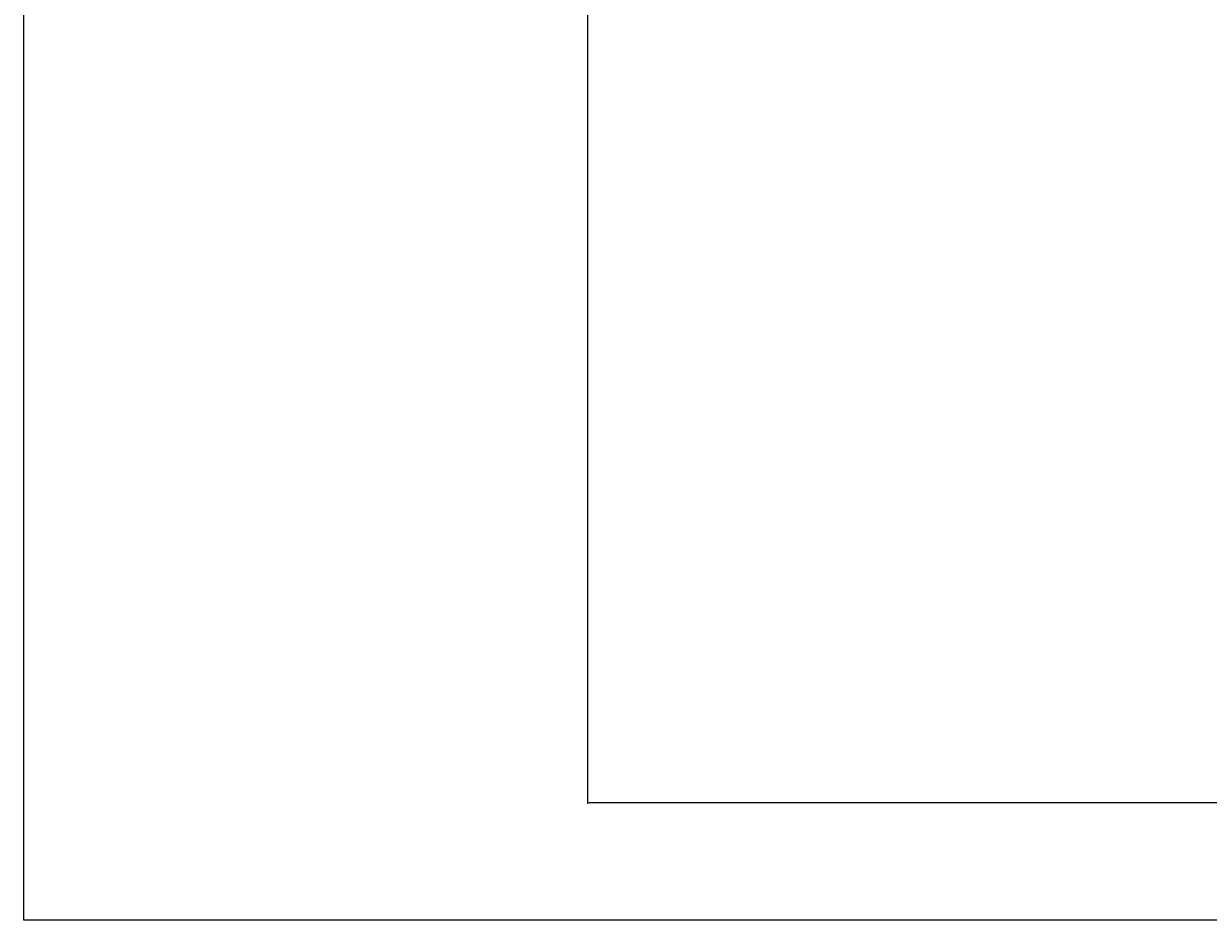
# Model space of a CAD drawing. Units: inches. Extents: x 1601 to 2297, y 1496 to 2631.
# Tile 1 of 57: x 1601 to 1780, y 1496 to 1632. Entities that reach past the tile are written whole.
import ezdxf

# ---------------------------------------------------------------- set-up
doc = ezdxf.new("R2010")
doc.units = ezdxf.units.IN
doc.layers.add('A-ANNO-DIMS', color=2, linetype='Continuous', lineweight=18)
doc.layers.add('A-ANNO-TTLB', color=7, linetype='Continuous', lineweight=25)
doc.styles.get("Standard").update_dxf_attribs({"font": 'arial.ttf'})
doc.dimstyles.get("Standard").update_dxf_attribs({"dimtxt": 0.18, "dimasz": 0.18, "dimexe": 0.18, "dimexo": 0.0625, "dimgap": 0.09, "dimtad": 0, "dimtih": 1, "dimtoh": 1, "dimdec": 4, "dimzin": 0, "dimdsep": 46, "dimtxsty": 'Standard', "dimcen": 0.09, "dimadec": 0, "dimazin": 0, "dimtfac": 1, "dimtdec": 4, "dimtofl": 0, "dimtmove": 0, "dimatfit": 3, "dimfxl": 1, "dimtolj": 1, "dimtzin": 0, "dimarcsym": 0})

# ---------------------------------------------------------------- blocks, each defined once
blk = doc.blocks.new('*D34')
at = {"layer": 'A-ANNO-DIMS', "color": 0, "lineweight": -2, "transparency": 16777216}
for p, q in [((1686.04, 1635.26), (1686.04, 1513.75)), ((1893.04, 1635.26), (1893.04, 1513.75)), ((1686.22, 1513.93), (1789.25, 1513.93)), ((1892.86, 1513.93), (1789.83, 1513.93))]:
    blk.add_line(p, q, dxfattribs=at)
at = {"layer": 'A-ANNO-DIMS', "color": 0, "transparency": 16777216}
for points in [[(1686.22, 1513.96), (1686.22, 1513.9), (1686.04, 1513.93)], [(1892.86, 1513.96), (1892.86, 1513.9), (1893.04, 1513.93)]]:
    blk.add_solid(points, dxfattribs=at)
at = {"layer": 'Defpoints', "color": 0, "transparency": 16777216}
for p in [(1686.04, 1635.33), (1893.04, 1635.33), (1893.04, 1513.93)]:
    blk.add_point(p, dxfattribs=at)
at = {"layer": 'A-ANNO-DIMS', "color": 0, "transparency": 16777216, "insert": (1789.54, 1513.93), "char_height": 0.18, "attachment_point": 5}
blk.add_mtext('\\A1;207', dxfattribs=at)

msp = doc.modelspace()

# ---------------------------------------------------------------- linework, layer by layer
at = {"layer": 'A-ANNO-TTLB'}
msp.add_lwpolyline([(1600.5933, 2631.1477), (2297.129, 2631.1477), (2297.129, 1496.1026), (1600.5933, 1496.1026)], close=True, dxfattribs=at)

# ---------------------------------------------------------------- dimensions: what is measured, and where the dimension line sits
at = {"layer": 'A-ANNO-DIMS'}
dim = msp.add_linear_dim(base=(1893.0373, 1513.9279), p1=(1686.0373, 1635.3254), p2=(1893.0373, 1635.3254), dimstyle='Standard', override={"dimdec": 0, "dimlfac": 1, "dimrnd": 0, "dimzin": 0, "dimdsep": 46, "dimlunit": 2}, dxfattribs=at)
dim.commit()
dim.dimension.update_dxf_attribs({"geometry": '*D34', "text_midpoint": (1789.5373, 1513.9279)})

doc.saveas('drawing.dxf')
